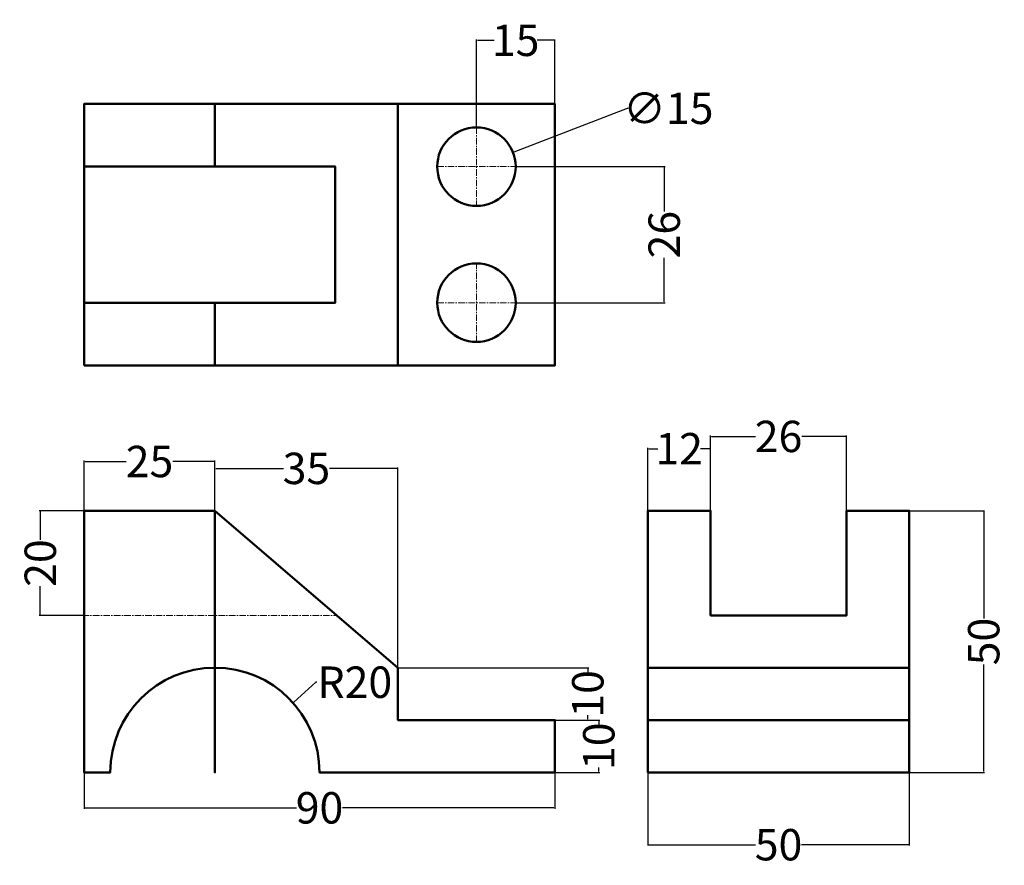
# Model space of a CAD drawing. Units: millimetres. Extents: x 0 to 188, y 20 to 181.
import ezdxf

# ---------------------------------------------------------------- set-up
doc = ezdxf.new("R2010")
doc.units = ezdxf.units.MM
doc.header["$MEASUREMENT"] = 0
doc.linetypes.add('CENTER', pattern=[2, 1.25, -0.25, 0.25, -0.25])
for name, color, linetype, lineweight in [('M-CNTR', 4, 'CENTER', 18), ('M-DIMS', 2, 'Continuous', 25), ('M-OUTL', 7, 'Continuous', 50)]:
    doc.layers.add(name, color=color, linetype=linetype, lineweight=lineweight)
doc.styles.get("Standard").update_dxf_attribs({"font": 'arial.ttf'})
doc.dimstyles.get("Standard").update_dxf_attribs({"dimtxt": 6, "dimasz": 0.18, "dimexe": 0.18, "dimexo": 0.0625, "dimgap": 0.09, "dimtad": 0, "dimtoh": 1, "dimdec": 0, "dimzin": 0, "dimdsep": 46, "dimtxsty": 'Standard', "dimcen": 0.09, "dimadec": 0, "dimazin": 0, "dimtfac": 1, "dimtdec": 0, "dimtofl": 0, "dimtmove": 0, "dimatfit": 3, "dimfxl": 1, "dimtolj": 1, "dimtzin": 0, "dimarcsym": 0})

# ---------------------------------------------------------------- blocks, each defined once
blk = doc.blocks.new('*D1')
at = {"layer": 'Defpoints', "color": 0, "transparency": 16777216}
for p in [(131.79, 99.14), (119.79, 87.29), (131.79, 87.29)]:
    blk.add_point(p, dxfattribs=at)
at = {"layer": 'M-DIMS', "color": 0, "lineweight": -2, "transparency": 16777216}
for p, q in [((119.79, 87.35), (119.79, 99.32)), ((119.97, 99.14), (121.72, 99.14)), ((131.61, 99.14), (129.87, 99.14)), ((131.79, 87.35), (131.79, 99.32))]:
    blk.add_line(p, q, dxfattribs=at)
at = {"layer": 'M-DIMS', "color": 0, "transparency": 16777216}
for points in [[(119.97, 99.17), (119.97, 99.11), (119.79, 99.14)], [(131.61, 99.17), (131.61, 99.11), (131.79, 99.14)]]:
    blk.add_solid(points, dxfattribs=at)
at = {"layer": 'M-DIMS', "color": 0, "transparency": 16777216, "insert": (125.79, 99.14), "char_height": 6, "attachment_point": 5}
blk.add_mtext('\\A1;12', dxfattribs=at)
blk = doc.blocks.new('*D2')
at = {"layer": 'Defpoints', "color": 0, "transparency": 16777216}
for p in [(157.79, 101.49), (131.79, 87.29), (157.79, 87.29)]:
    blk.add_point(p, dxfattribs=at)
at = {"layer": 'M-DIMS', "color": 0, "lineweight": -2, "transparency": 16777216}
for p, q in [((131.79, 87.35), (131.79, 101.67)), ((157.79, 87.35), (157.79, 101.67)), ((131.97, 101.49), (140.35, 101.49)), ((157.61, 101.49), (149.23, 101.49))]:
    blk.add_line(p, q, dxfattribs=at)
at = {"layer": 'M-DIMS', "color": 0, "transparency": 16777216}
for points in [[(131.97, 101.52), (131.97, 101.46), (131.79, 101.49)], [(157.61, 101.52), (157.61, 101.46), (157.79, 101.49)]]:
    blk.add_solid(points, dxfattribs=at)
at = {"layer": 'M-DIMS', "color": 0, "transparency": 16777216, "insert": (144.79, 101.49), "char_height": 6, "attachment_point": 5}
blk.add_mtext('\\A1;26', dxfattribs=at)
blk = doc.blocks.new('*D3')
at = {"layer": 'Defpoints', "color": 0, "transparency": 16777216}
for p in [(169.79, 87.29), (169.79, 37.29), (184.01, 37.29)]:
    blk.add_point(p, dxfattribs=at)
at = {"layer": 'M-DIMS', "color": 0, "lineweight": -2, "transparency": 16777216}
for p, q in [((169.85, 87.29), (184.19, 87.29)), ((184.01, 87.11), (184.01, 66.67)), ((184.01, 37.47), (184.01, 57.91)), ((169.85, 37.29), (184.19, 37.29))]:
    blk.add_line(p, q, dxfattribs=at)
at = {"layer": 'M-DIMS', "color": 0, "transparency": 16777216}
for points in [[(183.98, 87.11), (184.04, 87.11), (184.01, 87.29)], [(183.98, 37.47), (184.04, 37.47), (184.01, 37.29)]]:
    blk.add_solid(points, dxfattribs=at)
at = {"layer": 'M-DIMS', "color": 0, "transparency": 16777216, "insert": (184.01, 62.29), "char_height": 6, "attachment_point": 5, "rotation": 90}
blk.add_mtext('\\A1;50', dxfattribs=at)
blk = doc.blocks.new('*D4')
at = {"layer": 'Defpoints', "color": 0, "transparency": 16777216}
for p in [(119.79, 37.29), (169.79, 37.29), (169.79, 23.46)]:
    blk.add_point(p, dxfattribs=at)
at = {"layer": 'M-DIMS', "color": 0, "lineweight": -2, "transparency": 16777216}
for p, q in [((119.79, 37.23), (119.79, 23.28)), ((169.79, 37.23), (169.79, 23.28)), ((119.97, 23.46), (140.41, 23.46)), ((169.61, 23.46), (149.17, 23.46))]:
    blk.add_line(p, q, dxfattribs=at)
at = {"layer": 'M-DIMS', "color": 0, "transparency": 16777216}
for points in [[(119.97, 23.49), (119.97, 23.43), (119.79, 23.46)], [(169.61, 23.49), (169.61, 23.43), (169.79, 23.46)]]:
    blk.add_solid(points, dxfattribs=at)
at = {"layer": 'M-DIMS', "color": 0, "transparency": 16777216, "insert": (144.79, 23.46), "char_height": 6, "attachment_point": 5}
blk.add_mtext('\\A1;50', dxfattribs=at)
blk = doc.blocks.new('*D5')
at = {"layer": 'Defpoints', "color": 0, "transparency": 16777216}
for p in [(72.03, 57.29), (72.03, 47.29), (108.32, 47.29)]:
    blk.add_point(p, dxfattribs=at)
at = {"layer": 'M-DIMS', "color": 0, "lineweight": -2, "transparency": 16777216}
for p, q in [((72.09, 57.29), (108.5, 57.29)), ((108.32, 57.11), (108.32, 56.38)), ((72.09, 47.29), (108.5, 47.29)), ((108.32, 47.47), (108.32, 48.19))]:
    blk.add_line(p, q, dxfattribs=at)
at = {"layer": 'M-DIMS', "color": 0, "transparency": 16777216}
for points in [[(108.29, 57.11), (108.35, 57.11), (108.32, 57.29)], [(108.29, 47.47), (108.35, 47.47), (108.32, 47.29)]]:
    blk.add_solid(points, dxfattribs=at)
at = {"layer": 'M-DIMS', "color": 0, "transparency": 16777216, "insert": (108.32, 52.29), "char_height": 6, "attachment_point": 5, "rotation": 90}
blk.add_mtext('\\A1;10', dxfattribs=at)
blk = doc.blocks.new('*D6')
at = {"layer": 'Defpoints', "color": 0, "transparency": 16777216}
for p in [(102.03, 47.29), (102.03, 37.29), (110.42, 37.29)]:
    blk.add_point(p, dxfattribs=at)
at = {"layer": 'M-DIMS', "color": 0, "lineweight": -2, "transparency": 16777216}
for p, q in [((102.09, 47.29), (110.6, 47.29)), ((110.42, 47.11), (110.42, 46.38)), ((110.42, 37.47), (110.42, 38.19)), ((102.09, 37.29), (110.6, 37.29))]:
    blk.add_line(p, q, dxfattribs=at)
at = {"layer": 'M-DIMS', "color": 0, "transparency": 16777216}
for points in [[(110.39, 47.11), (110.45, 47.11), (110.42, 47.29)], [(110.39, 37.47), (110.45, 37.47), (110.42, 37.29)]]:
    blk.add_solid(points, dxfattribs=at)
at = {"layer": 'M-DIMS', "color": 0, "transparency": 16777216, "insert": (110.42, 42.29), "char_height": 6, "attachment_point": 5, "rotation": 90}
blk.add_mtext('\\A1;10', dxfattribs=at)
blk = doc.blocks.new('*D7')
at = {"layer": 'Defpoints', "color": 0, "transparency": 16777216}
for p in [(12.03, 37.68), (102.03, 37.29), (102.03, 30.51)]:
    blk.add_point(p, dxfattribs=at)
at = {"layer": 'M-DIMS', "color": 0, "lineweight": -2, "transparency": 16777216}
for p, q in [((12.03, 37.62), (12.03, 30.33)), ((102.03, 37.23), (102.03, 30.33)), ((12.21, 30.51), (52.65, 30.51)), ((101.85, 30.51), (61.4, 30.51))]:
    blk.add_line(p, q, dxfattribs=at)
at = {"layer": 'M-DIMS', "color": 0, "transparency": 16777216}
for points in [[(12.21, 30.54), (12.21, 30.48), (12.03, 30.51)], [(101.85, 30.54), (101.85, 30.48), (102.03, 30.51)]]:
    blk.add_solid(points, dxfattribs=at)
at = {"layer": 'M-DIMS', "color": 0, "transparency": 16777216, "insert": (57.03, 30.51), "char_height": 6, "attachment_point": 5}
blk.add_mtext('\\A1;90', dxfattribs=at)
blk = doc.blocks.new('*D8')
at = {"layer": 'Defpoints', "color": 0, "transparency": 16777216}
for p in [(12.03, 87.29), (3.64, 67.29), (12.03, 67.29)]:
    blk.add_point(p, dxfattribs=at)
at = {"layer": 'M-DIMS', "color": 0, "lineweight": -2, "transparency": 16777216}
for p, q in [((11.96, 87.29), (3.46, 87.29)), ((3.64, 87.11), (3.64, 81.72)), ((3.64, 67.47), (3.64, 72.86)), ((11.96, 67.29), (3.46, 67.29))]:
    blk.add_line(p, q, dxfattribs=at)
at = {"layer": 'M-DIMS', "color": 0, "transparency": 16777216}
for points in [[(3.61, 87.11), (3.67, 87.11), (3.64, 87.29)], [(3.61, 67.47), (3.67, 67.47), (3.64, 67.29)]]:
    blk.add_solid(points, dxfattribs=at)
at = {"layer": 'M-DIMS', "color": 0, "transparency": 16777216, "insert": (3.64, 77.29), "char_height": 6, "attachment_point": 5, "rotation": 90}
blk.add_mtext('\\A1;20', dxfattribs=at)
blk = doc.blocks.new('*D9')
at = {"layer": 'Defpoints', "color": 0, "transparency": 16777216}
for p in [(37.03, 96.7), (12.03, 87.29), (37.03, 87.29)]:
    blk.add_point(p, dxfattribs=at)
at = {"layer": 'M-DIMS', "color": 0, "lineweight": -2, "transparency": 16777216}
for p, q in [((12.03, 87.35), (12.03, 96.88)), ((12.21, 96.7), (20.07, 96.7)), ((36.85, 96.7), (28.99, 96.7)), ((37.03, 87.35), (37.03, 96.88))]:
    blk.add_line(p, q, dxfattribs=at)
at = {"layer": 'M-DIMS', "color": 0, "transparency": 16777216}
for points in [[(12.21, 96.73), (12.21, 96.67), (12.03, 96.7)], [(36.85, 96.73), (36.85, 96.67), (37.03, 96.7)]]:
    blk.add_solid(points, dxfattribs=at)
at = {"layer": 'M-DIMS', "color": 0, "transparency": 16777216, "insert": (24.53, 96.7), "char_height": 6, "attachment_point": 5}
blk.add_mtext('\\A1;25', dxfattribs=at)
blk = doc.blocks.new('*D10')
at = {"layer": 'Defpoints', "color": 0, "transparency": 16777216}
for p in [(72.03, 95.38), (37.03, 92.11), (72.03, 57.29)]:
    blk.add_point(p, dxfattribs=at)
at = {"layer": 'M-DIMS', "color": 0, "lineweight": -2, "transparency": 16777216}
for p, q in [((37.03, 92.18), (37.03, 95.56)), ((37.21, 95.38), (50.12, 95.38)), ((71.85, 95.38), (58.93, 95.38)), ((72.03, 57.35), (72.03, 95.56))]:
    blk.add_line(p, q, dxfattribs=at)
at = {"layer": 'M-DIMS', "color": 0, "transparency": 16777216}
for points in [[(37.21, 95.41), (37.21, 95.35), (37.03, 95.38)], [(71.85, 95.41), (71.85, 95.35), (72.03, 95.38)]]:
    blk.add_solid(points, dxfattribs=at)
at = {"layer": 'M-DIMS', "color": 0, "transparency": 16777216, "insert": (54.53, 95.38), "char_height": 6, "attachment_point": 5}
blk.add_mtext('\\A1;35', dxfattribs=at)
blk = doc.blocks.new('*D11')
at = {"layer": 'Defpoints', "color": 0, "transparency": 16777216}
for p in [(51.95, 50.6), (37.03, 37.29)]:
    blk.add_point(p, dxfattribs=at)
at = {"layer": 'M-DIMS', "color": 0, "lineweight": -2, "transparency": 16777216}
for p, q in [((56.35, 54.52), (52.09, 50.72)), ((56.53, 54.52), (56.35, 54.52)), ((36.94, 37.29), (37.12, 37.29)), ((37.03, 37.2), (37.03, 37.38))]:
    blk.add_line(p, q, dxfattribs=at)
at = {"layer": 'M-DIMS', "color": 0, "transparency": 16777216}
blk.add_solid([(52.07, 50.74), (52.11, 50.7), (51.95, 50.6)], dxfattribs=at)
at = {"layer": 'M-DIMS', "color": 0, "transparency": 16777216, "insert": (63.78, 54.52), "char_height": 6, "attachment_point": 5}
blk.add_mtext('\\A1;R20', dxfattribs=at)
blk = doc.blocks.new('*D12')
at = {"layer": 'Defpoints', "color": 0, "transparency": 16777216}
for p in [(102.03, 177.19), (102.03, 165.05), (87.03, 160.55)]:
    blk.add_point(p, dxfattribs=at)
at = {"layer": 'M-DIMS', "color": 0, "lineweight": -2, "transparency": 16777216}
for p, q in [((87.03, 160.61), (87.03, 177.37)), ((87.21, 177.19), (90.4, 177.19)), ((101.85, 177.19), (98.65, 177.19)), ((102.03, 165.11), (102.03, 177.37))]:
    blk.add_line(p, q, dxfattribs=at)
at = {"layer": 'M-DIMS', "color": 0, "transparency": 16777216}
for points in [[(87.21, 177.22), (87.21, 177.16), (87.03, 177.19)], [(101.85, 177.22), (101.85, 177.16), (102.03, 177.19)]]:
    blk.add_solid(points, dxfattribs=at)
at = {"layer": 'M-DIMS', "color": 0, "transparency": 16777216, "insert": (94.53, 177.19), "char_height": 6, "attachment_point": 5}
blk.add_mtext('\\A1;15', dxfattribs=at)
blk = doc.blocks.new('*D13')
at = {"layer": 'Defpoints', "color": 0, "transparency": 16777216}
for p in [(94.53, 153.05), (94.53, 127.05), (122.92, 127.05)]:
    blk.add_point(p, dxfattribs=at)
at = {"layer": 'M-DIMS', "color": 0, "lineweight": -2, "transparency": 16777216}
for p, q in [((94.59, 153.05), (123.1, 153.05)), ((122.92, 152.87), (122.92, 144.49)), ((122.92, 127.23), (122.92, 135.61)), ((94.59, 127.05), (123.1, 127.05))]:
    blk.add_line(p, q, dxfattribs=at)
at = {"layer": 'M-DIMS', "color": 0, "transparency": 16777216}
for points in [[(122.89, 152.87), (122.95, 152.87), (122.92, 153.05)], [(122.89, 127.23), (122.95, 127.23), (122.92, 127.05)]]:
    blk.add_solid(points, dxfattribs=at)
at = {"layer": 'M-DIMS', "color": 0, "transparency": 16777216, "insert": (122.92, 140.05), "char_height": 6, "attachment_point": 5, "rotation": 90}
blk.add_mtext('\\A1;26', dxfattribs=at)
blk = doc.blocks.new('*D14')
at = {"layer": 'Defpoints', "color": 0, "transparency": 16777216}
for p in [(94.02, 155.75), (80.03, 150.34)]:
    blk.add_point(p, dxfattribs=at)
at = {"layer": 'M-DIMS', "color": 0, "lineweight": -2, "transparency": 16777216}
for p, q in [((115.85, 164.19), (94.19, 155.82)), ((116.03, 164.19), (115.85, 164.19)), ((86.94, 153.05), (87.12, 153.05)), ((87.03, 152.96), (87.03, 153.14))]:
    blk.add_line(p, q, dxfattribs=at)
at = {"layer": 'M-DIMS', "color": 0, "transparency": 16777216}
blk.add_solid([(94.18, 155.85), (94.2, 155.79), (94.02, 155.75)], dxfattribs=at)
at = {"layer": 'M-DIMS', "color": 0, "transparency": 16777216, "insert": (123.71, 164.19), "char_height": 6, "attachment_point": 5}
blk.add_mtext('\\A1;∅15', dxfattribs=at)

msp = doc.modelspace()

# ---------------------------------------------------------------- linework, layer by layer
at = {"layer": 'M-CNTR'}
for p, q in [((87.03, 160.55), (87.03, 145.55)), ((79.53, 153.05), (94.53, 153.05)), ((87.03, 119.55), (87.03, 134.55)), ((79.53, 127.05), (94.53, 127.05)), ((7.71, 67.29), (60.36, 67.29))]:
    msp.add_line(p, q, dxfattribs=at)
at = {"layer": 'M-OUTL'}
for p, q in [((37.03, 153.05), (37.03, 165.05)), ((72.03, 115.05), (72.03, 165.05)), ((37.03, 115.05), (37.03, 127.05)), ((119.79, 57.29), (169.79, 57.29)), ((119.79, 47.29), (169.79, 47.29))]:
    msp.add_line(p, q, dxfattribs=at)
for points in [[(12.03, 115.05), (12.03, 165.05), (102.03, 165.05), (102.03, 115.05)], [(119.79, 37.29), (169.79, 37.29), (169.79, 87.29), (157.79, 87.29), (157.79, 67.29), (131.79, 67.29), (131.79, 87.29), (119.79, 87.29)]]:
    msp.add_lwpolyline(points, close=True, dxfattribs=at)
msp.add_lwpolyline([(12.03, 127.05), (60.03, 127.05), (60.03, 153.05), (12.03, 153.05)], dxfattribs=at)
msp.add_lwpolyline([(37.03, 87.29), (72.03, 57.29), (72.03, 47.29), (102.03, 47.29), (102.03, 37.29), (57.03, 37.29, 1), (17.03, 37.29), (12.03, 37.29), (12.03, 87.29), (37.03, 87.29), (37.03, 37.29)], format="xyb", dxfattribs=at)
for centre in [(87.03, 153.05), (87.03, 127.05)]:
    msp.add_circle(centre, 7.5, dxfattribs=at)

# ---------------------------------------------------------------- dimensions: what is measured, and where the dimension line sits
at = {"layer": 'M-DIMS'}
for base, p1, p2, picture, middle in [((102.03, 177.19), (87.03, 160.55), (102.03, 165.05), '*D12', (94.53, 177.19)), ((157.79, 101.49), (131.79, 87.29), (157.79, 87.29), '*D2', (144.79, 101.49)), ((131.79, 99.14), (119.79, 87.29), (131.79, 87.29), '*D1', (125.79, 99.14)), ((37.03, 96.7), (12.03, 87.29), (37.03, 87.29), '*D9', (24.53, 96.7)), ((72.03, 95.38), (37.03, 92.11), (72.03, 57.29), '*D10', (54.53, 95.38)), ((102.03, 30.51), (12.03, 37.68), (102.03, 37.29), '*D7', (57.03, 30.51)), ((169.79, 23.46), (119.79, 37.29), (169.79, 37.29), '*D4', (144.79, 23.46))]:
    dim = msp.add_linear_dim(base=base, p1=p1, p2=p2, dimstyle='Standard', override={"dimclrd": 0, "dimclre": 0, "dimclrt": 0}, dxfattribs=at)
    dim.commit()
    dim.dimension.update_dxf_attribs({"geometry": picture, "text_midpoint": middle})
dim = msp.add_diameter_dim_2p(p1=(80.03, 150.34), p2=(94.02, 155.75), dimstyle='Standard', override={"dimclrd": 0, "dimclre": 0, "dimclrt": 0}, dxfattribs=at)
dim.commit()
dim.dimension.update_dxf_attribs({"geometry": '*D14', "text_midpoint": (123.71, 164.19), "dimtype": 163})
for base, p1, p2, picture, middle in [((122.92, 127.05), (94.53, 153.05), (94.53, 127.05), '*D13', (122.92, 140.05)), ((3.64, 67.29), (12.03, 87.29), (12.03, 67.29), '*D8', (3.64, 77.29)), ((184.01, 37.29), (169.79, 87.29), (169.79, 37.29), '*D3', (184.01, 62.29)), ((108.32, 47.29), (72.03, 57.29), (72.03, 47.29), '*D5', (108.32, 52.29)), ((110.42, 37.29), (102.03, 47.29), (102.03, 37.29), '*D6', (110.42, 42.29))]:
    dim = msp.add_linear_dim(base=base, p1=p1, p2=p2, angle=90, dimstyle='Standard', override={"dimclrd": 0, "dimclre": 0, "dimclrt": 0}, dxfattribs=at)
    dim.commit()
    dim.dimension.update_dxf_attribs({"geometry": picture, "text_midpoint": middle})
dim = msp.add_radius_dim(center=(37.03, 37.29), mpoint=(51.95, 50.6), dimstyle='Standard', override={"dimclrd": 0, "dimclre": 0, "dimclrt": 0}, dxfattribs=at)
dim.commit()
dim.dimension.update_dxf_attribs({"geometry": '*D11', "text_midpoint": (63.78, 54.52), "dimtype": 164})

doc.saveas('drawing.dxf')
